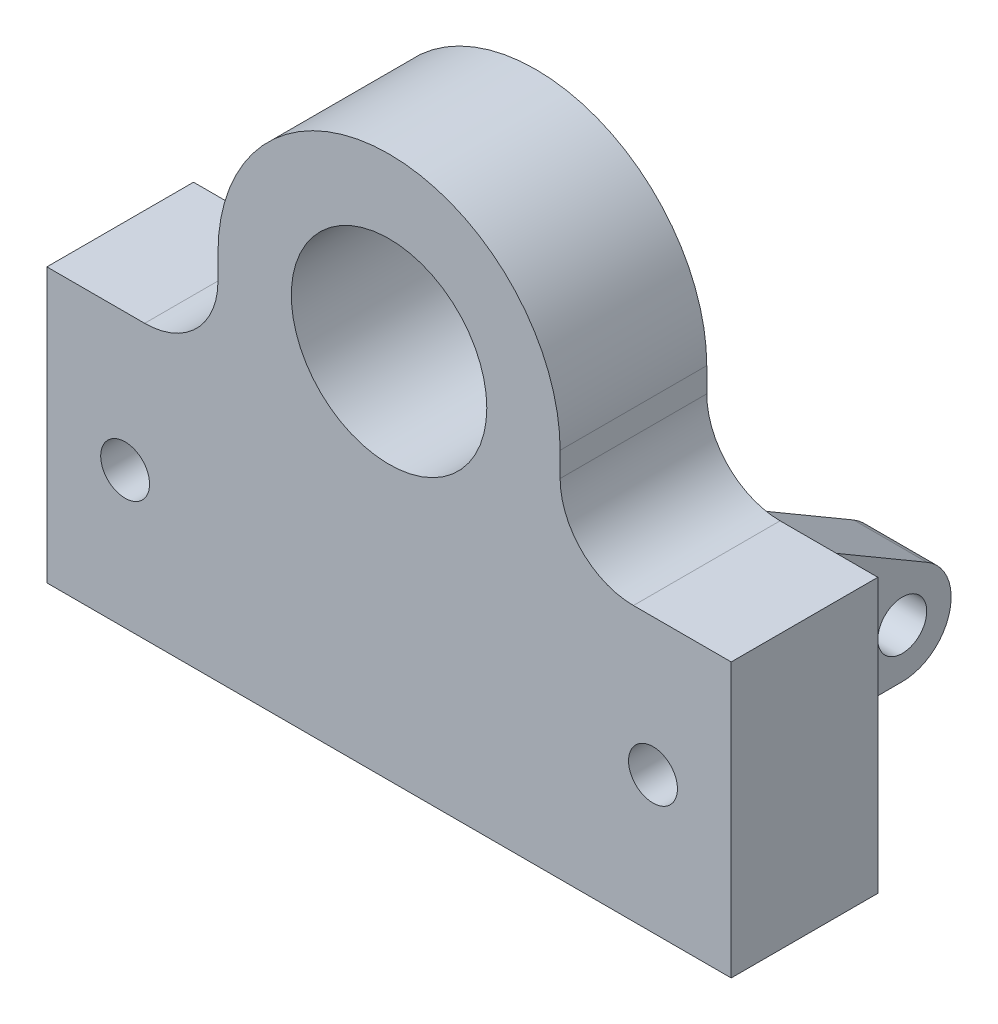
ISO-10303-21;
HEADER;
FILE_DESCRIPTION(('STEP AP214'),'2;1');
FILE_NAME('part.step','',(''),(''),'','','');
FILE_SCHEMA(('AUTOMOTIVE_DESIGN { 1 0 10303 214 1 1 1 1 }'));
ENDSEC;
DATA;
#1=APPLICATION_CONTEXT('core data for automotive mechanical design processes');
#2=APPLICATION_PROTOCOL_DEFINITION('international standard','automotive_design',2000,#1);
#3=PRODUCT_CONTEXT('',#1,'mechanical');
#4=PRODUCT('Part','Part','',(#3));
#5=PRODUCT_RELATED_PRODUCT_CATEGORY('part','',(#4));
#6=PRODUCT_DEFINITION_FORMATION('','',#4);
#7=PRODUCT_DEFINITION_CONTEXT('part definition',#1,'design');
#8=PRODUCT_DEFINITION('design','',#6,#7);
#9=PRODUCT_DEFINITION_SHAPE('','',#8);
#10=(LENGTH_UNIT() NAMED_UNIT(*) SI_UNIT(.MILLI.,.METRE.));
#11=(NAMED_UNIT(*) PLANE_ANGLE_UNIT() SI_UNIT($,.RADIAN.));
#12=(NAMED_UNIT(*) SI_UNIT($,.STERADIAN.) SOLID_ANGLE_UNIT());
#13=UNCERTAINTY_MEASURE_WITH_UNIT(LENGTH_MEASURE(1.E-05),#10,'distance_accuracy_value','');
#14=(GEOMETRIC_REPRESENTATION_CONTEXT(3) GLOBAL_UNCERTAINTY_ASSIGNED_CONTEXT((#13)) GLOBAL_UNIT_ASSIGNED_CONTEXT((#10,
#11,#12)) REPRESENTATION_CONTEXT('',''));
#15=CARTESIAN_POINT('',(0.,0.,0.));
#16=DIRECTION('',(0.,0.,1.));
#17=DIRECTION('',(1.,0.,0.));
#18=AXIS2_PLACEMENT_3D('',#15,#16,#17);
#19=CARTESIAN_POINT('',(0.,0.,30.));
#20=DIRECTION('',(0.,1.,0.));
#21=DIRECTION('',(0.,0.,1.));
#22=AXIS2_PLACEMENT_3D('',#19,#20,#21);
#23=PLANE('',#22);
#24=DIRECTION('',(1.,0.,0.));
#25=VECTOR('',#24,1.);
#26=CARTESIAN_POINT('',(0.,0.,0.));
#27=LINE('',#26,#25);
#28=CARTESIAN_POINT('',(0.,0.,0.));
#29=VERTEX_POINT('',#28);
#30=CARTESIAN_POINT('',(35.,0.,0.));
#31=VERTEX_POINT('',#30);
#32=EDGE_CURVE('E251',#29,#31,#27,.T.);
#33=ORIENTED_EDGE('',*,*,#32,.T.);
#34=DIRECTION('',(0.,0.,-1.));
#35=VECTOR('',#34,1.);
#36=CARTESIAN_POINT('',(35.,0.,0.));
#37=LINE('',#36,#35);
#38=CARTESIAN_POINT('',(35.,0.,-40.));
#39=VERTEX_POINT('',#38);
#40=EDGE_CURVE('E189',#31,#39,#37,.T.);
#41=ORIENTED_EDGE('',*,*,#40,.T.);
#42=DIRECTION('',(-1.,0.,0.));
#43=VECTOR('',#42,1.);
#44=CARTESIAN_POINT('',(50.,0.,-40.));
#45=LINE('',#44,#43);
#46=CARTESIAN_POINT('',(50.,0.,-40.));
#47=VERTEX_POINT('',#46);
#48=EDGE_CURVE('E222',#47,#39,#45,.T.);
#49=ORIENTED_EDGE('',*,*,#48,.F.);
#50=DIRECTION('',(0.,0.,-1.));
#51=VECTOR('',#50,1.);
#52=CARTESIAN_POINT('',(50.,0.,0.));
#53=LINE('',#52,#51);
#54=CARTESIAN_POINT('',(50.,0.,0.));
#55=VERTEX_POINT('',#54);
#56=EDGE_CURVE('E200',#55,#47,#53,.T.);
#57=ORIENTED_EDGE('',*,*,#56,.F.);
#58=CARTESIAN_POINT('',(90.,0.,0.));
#59=VERTEX_POINT('',#58);
#60=EDGE_CURVE('E258',#55,#59,#27,.T.);
#61=ORIENTED_EDGE('',*,*,#60,.T.);
#62=DIRECTION('',(0.,0.,-1.));
#63=VECTOR('',#62,1.);
#64=CARTESIAN_POINT('',(90.,0.,0.));
#65=LINE('',#64,#63);
#66=CARTESIAN_POINT('',(90.,0.,-40.));
#67=VERTEX_POINT('',#66);
#68=EDGE_CURVE('E187',#59,#67,#65,.T.);
#69=ORIENTED_EDGE('',*,*,#68,.T.);
#70=DIRECTION('',(-1.,0.,0.));
#71=VECTOR('',#70,1.);
#72=CARTESIAN_POINT('',(105.,0.,-40.));
#73=LINE('',#72,#71);
#74=CARTESIAN_POINT('',(105.,0.,-40.));
#75=VERTEX_POINT('',#74);
#76=EDGE_CURVE('E175',#75,#67,#73,.T.);
#77=ORIENTED_EDGE('',*,*,#76,.F.);
#78=DIRECTION('',(0.,0.,-1.));
#79=VECTOR('',#78,1.);
#80=CARTESIAN_POINT('',(105.,0.,0.));
#81=LINE('',#80,#79);
#82=CARTESIAN_POINT('',(105.,0.,0.));
#83=VERTEX_POINT('',#82);
#84=EDGE_CURVE('E177',#83,#75,#81,.T.);
#85=ORIENTED_EDGE('',*,*,#84,.F.);
#86=CARTESIAN_POINT('',(140.,0.,0.));
#87=VERTEX_POINT('',#86);
#88=EDGE_CURVE('E64',#83,#87,#27,.T.);
#89=ORIENTED_EDGE('',*,*,#88,.T.);
#90=DIRECTION('',(0.,0.,-1.));
#91=VECTOR('',#90,1.);
#92=CARTESIAN_POINT('',(140.,0.,30.));
#93=LINE('',#92,#91);
#94=CARTESIAN_POINT('',(140.,0.,30.));
#95=VERTEX_POINT('',#94);
#96=EDGE_CURVE('E11',#95,#87,#93,.T.);
#97=ORIENTED_EDGE('',*,*,#96,.F.);
#98=DIRECTION('',(1.,0.,0.));
#99=VECTOR('',#98,1.);
#100=CARTESIAN_POINT('',(0.,0.,30.));
#101=LINE('',#100,#99);
#102=CARTESIAN_POINT('',(0.,0.,30.));
#103=VERTEX_POINT('',#102);
#104=EDGE_CURVE('E229',#103,#95,#101,.T.);
#105=ORIENTED_EDGE('',*,*,#104,.F.);
#106=DIRECTION('',(0.,0.,-1.));
#107=VECTOR('',#106,1.);
#108=CARTESIAN_POINT('',(0.,0.,30.));
#109=LINE('',#108,#107);
#110=EDGE_CURVE('E252',#103,#29,#109,.T.);
#111=ORIENTED_EDGE('',*,*,#110,.T.);
#112=EDGE_LOOP('',(#33,#41,#49,#57,#61,#69,#77,#85,#89,#97,#105,#111));
#113=FACE_BOUND('',#112,.T.);
#114=ADVANCED_FACE('F44',(#113),#23,.F.);
#115=CARTESIAN_POINT('',(140.,0.,30.));
#116=DIRECTION('',(-1.,0.,0.));
#117=DIRECTION('',(0.,0.,1.));
#118=AXIS2_PLACEMENT_3D('',#115,#116,#117);
#119=PLANE('',#118);
#120=DIRECTION('',(0.,1.,0.));
#121=VECTOR('',#120,1.);
#122=CARTESIAN_POINT('',(140.,0.,0.));
#123=LINE('',#122,#121);
#124=CARTESIAN_POINT('',(140.,56.,0.));
#125=VERTEX_POINT('',#124);
#126=EDGE_CURVE('E254',#87,#125,#123,.T.);
#127=ORIENTED_EDGE('',*,*,#126,.T.);
#128=DIRECTION('',(0.,0.,-1.));
#129=VECTOR('',#128,1.);
#130=CARTESIAN_POINT('',(140.,56.,30.));
#131=LINE('',#130,#129);
#132=CARTESIAN_POINT('',(140.,56.,30.));
#133=VERTEX_POINT('',#132);
#134=EDGE_CURVE('E52',#133,#125,#131,.T.);
#135=ORIENTED_EDGE('',*,*,#134,.F.);
#136=DIRECTION('',(0.,1.,0.));
#137=VECTOR('',#136,1.);
#138=CARTESIAN_POINT('',(140.,0.,30.));
#139=LINE('',#138,#137);
#140=EDGE_CURVE('E231',#95,#133,#139,.T.);
#141=ORIENTED_EDGE('',*,*,#140,.F.);
#142=ORIENTED_EDGE('',*,*,#96,.T.);
#143=EDGE_LOOP('',(#127,#135,#141,#142));
#144=FACE_BOUND('',#143,.T.);
#145=ADVANCED_FACE('F302',(#144),#119,.F.);
#146=CARTESIAN_POINT('',(125.,56.,30.));
#147=DIRECTION('',(0.,-1.,0.));
#148=DIRECTION('',(0.,0.,-1.));
#149=AXIS2_PLACEMENT_3D('',#146,#147,#148);
#150=PLANE('',#149);
#151=DIRECTION('',(-1.,0.,0.));
#152=VECTOR('',#151,1.);
#153=CARTESIAN_POINT('',(125.,56.,0.));
#154=LINE('',#153,#152);
#155=CARTESIAN_POINT('',(120.,56.,0.));
#156=VERTEX_POINT('',#155);
#157=EDGE_CURVE('E259',#125,#156,#154,.T.);
#158=ORIENTED_EDGE('',*,*,#157,.T.);
#159=DIRECTION('',(0.,0.,-1.));
#160=VECTOR('',#159,1.);
#161=CARTESIAN_POINT('',(120.,56.,30.));
#162=LINE('',#161,#160);
#163=CARTESIAN_POINT('',(120.,56.,30.));
#164=VERTEX_POINT('',#163);
#165=EDGE_CURVE('E294',#164,#156,#162,.T.);
#166=ORIENTED_EDGE('',*,*,#165,.F.);
#167=DIRECTION('',(-1.,0.,0.));
#168=VECTOR('',#167,1.);
#169=CARTESIAN_POINT('',(140.,56.,30.));
#170=LINE('',#169,#168);
#171=EDGE_CURVE('E237',#133,#164,#170,.T.);
#172=ORIENTED_EDGE('',*,*,#171,.F.);
#173=ORIENTED_EDGE('',*,*,#134,.T.);
#174=EDGE_LOOP('',(#158,#166,#172,#173));
#175=FACE_BOUND('',#174,.T.);
#176=ADVANCED_FACE('F303',(#175),#150,.F.);
#177=CARTESIAN_POINT('',(120.,71.,30.));
#178=DIRECTION('',(0.,0.,-1.));
#179=DIRECTION('',(-1.,0.,0.));
#180=AXIS2_PLACEMENT_3D('',#177,#178,#179);
#181=CYLINDRICAL_SURFACE('',#180,15.);
#182=CARTESIAN_POINT('',(120.,71.,0.));
#183=DIRECTION('',(0.,0.,-1.));
#184=DIRECTION('',(1.,0.,0.));
#185=AXIS2_PLACEMENT_3D('',#182,#183,#184);
#186=CIRCLE('',#185,15.);
#187=CARTESIAN_POINT('',(105.,71.,0.));
#188=VERTEX_POINT('',#187);
#189=EDGE_CURVE('E261',#156,#188,#186,.T.);
#190=ORIENTED_EDGE('',*,*,#189,.T.);
#191=DIRECTION('',(0.,0.,-1.));
#192=VECTOR('',#191,1.);
#193=CARTESIAN_POINT('',(105.,71.,30.));
#194=LINE('',#193,#192);
#195=CARTESIAN_POINT('',(105.,71.,30.));
#196=VERTEX_POINT('',#195);
#197=EDGE_CURVE('E292',#196,#188,#194,.T.);
#198=ORIENTED_EDGE('',*,*,#197,.F.);
#199=CARTESIAN_POINT('',(120.,71.,30.));
#200=DIRECTION('',(0.,0.,-1.));
#201=DIRECTION('',(1.,0.,0.));
#202=AXIS2_PLACEMENT_3D('',#199,#200,#201);
#203=CIRCLE('',#202,15.);
#204=EDGE_CURVE('E236',#164,#196,#203,.T.);
#205=ORIENTED_EDGE('',*,*,#204,.F.);
#206=ORIENTED_EDGE('',*,*,#165,.T.);
#207=EDGE_LOOP('',(#190,#198,#205,#206));
#208=FACE_BOUND('',#207,.T.);
#209=ADVANCED_FACE('F311',(#208),#181,.F.);
#210=CARTESIAN_POINT('',(105.,71.,30.));
#211=DIRECTION('',(-1.,0.,0.));
#212=DIRECTION('',(0.,-1.,0.));
#213=AXIS2_PLACEMENT_3D('',#210,#211,#212);
#214=PLANE('',#213);
#215=DIRECTION('',(0.,1.,0.));
#216=VECTOR('',#215,1.);
#217=CARTESIAN_POINT('',(105.,71.,0.));
#218=LINE('',#217,#216);
#219=CARTESIAN_POINT('',(105.,76.,0.));
#220=VERTEX_POINT('',#219);
#221=EDGE_CURVE('E263',#188,#220,#218,.T.);
#222=ORIENTED_EDGE('',*,*,#221,.T.);
#223=DIRECTION('',(0.,0.,-1.));
#224=VECTOR('',#223,1.);
#225=CARTESIAN_POINT('',(105.,76.,30.));
#226=LINE('',#225,#224);
#227=CARTESIAN_POINT('',(105.,76.,30.));
#228=VERTEX_POINT('',#227);
#229=EDGE_CURVE('E286',#228,#220,#226,.T.);
#230=ORIENTED_EDGE('',*,*,#229,.F.);
#231=DIRECTION('',(0.,1.,0.));
#232=VECTOR('',#231,1.);
#233=CARTESIAN_POINT('',(105.,71.,30.));
#234=LINE('',#233,#232);
#235=EDGE_CURVE('E238',#196,#228,#234,.T.);
#236=ORIENTED_EDGE('',*,*,#235,.F.);
#237=ORIENTED_EDGE('',*,*,#197,.T.);
#238=EDGE_LOOP('',(#222,#230,#236,#237));
#239=FACE_BOUND('',#238,.T.);
#240=ADVANCED_FACE('F320',(#239),#214,.F.);
#241=CARTESIAN_POINT('',(70.,76.,30.));
#242=DIRECTION('',(0.,0.,-1.));
#243=DIRECTION('',(-1.,0.,0.));
#244=AXIS2_PLACEMENT_3D('',#241,#242,#243);
#245=CYLINDRICAL_SURFACE('',#244,35.);
#246=CARTESIAN_POINT('',(70.,76.,0.));
#247=DIRECTION('',(0.,0.,1.));
#248=DIRECTION('',(1.,0.,0.));
#249=AXIS2_PLACEMENT_3D('',#246,#247,#248);
#250=CIRCLE('',#249,35.);
#251=CARTESIAN_POINT('',(35.,76.,0.));
#252=VERTEX_POINT('',#251);
#253=EDGE_CURVE('E264',#220,#252,#250,.T.);
#254=ORIENTED_EDGE('',*,*,#253,.T.);
#255=DIRECTION('',(0.,0.,-1.));
#256=VECTOR('',#255,1.);
#257=CARTESIAN_POINT('',(35.,76.,30.));
#258=LINE('',#257,#256);
#259=CARTESIAN_POINT('',(35.,76.,30.));
#260=VERTEX_POINT('',#259);
#261=EDGE_CURVE('E284',#260,#252,#258,.T.);
#262=ORIENTED_EDGE('',*,*,#261,.F.);
#263=CARTESIAN_POINT('',(70.,76.,30.));
#264=DIRECTION('',(0.,0.,1.));
#265=DIRECTION('',(1.,0.,0.));
#266=AXIS2_PLACEMENT_3D('',#263,#264,#265);
#267=CIRCLE('',#266,35.);
#268=EDGE_CURVE('E245',#228,#260,#267,.T.);
#269=ORIENTED_EDGE('',*,*,#268,.F.);
#270=ORIENTED_EDGE('',*,*,#229,.T.);
#271=EDGE_LOOP('',(#254,#262,#269,#270));
#272=FACE_BOUND('',#271,.T.);
#273=ADVANCED_FACE('F405',(#272),#245,.T.);
#274=CARTESIAN_POINT('',(35.,71.,30.));
#275=DIRECTION('',(1.,0.,0.));
#276=DIRECTION('',(0.,1.,0.));
#277=AXIS2_PLACEMENT_3D('',#274,#275,#276);
#278=PLANE('',#277);
#279=DIRECTION('',(0.,-1.,0.));
#280=VECTOR('',#279,1.);
#281=CARTESIAN_POINT('',(35.,71.,0.));
#282=LINE('',#281,#280);
#283=CARTESIAN_POINT('',(35.,71.,0.));
#284=VERTEX_POINT('',#283);
#285=EDGE_CURVE('E270',#252,#284,#282,.T.);
#286=ORIENTED_EDGE('',*,*,#285,.T.);
#287=DIRECTION('',(0.,0.,-1.));
#288=VECTOR('',#287,1.);
#289=CARTESIAN_POINT('',(35.,71.,30.));
#290=LINE('',#289,#288);
#291=CARTESIAN_POINT('',(35.,71.,30.));
#292=VERTEX_POINT('',#291);
#293=EDGE_CURVE('E285',#292,#284,#290,.T.);
#294=ORIENTED_EDGE('',*,*,#293,.F.);
#295=DIRECTION('',(0.,-1.,0.));
#296=VECTOR('',#295,1.);
#297=CARTESIAN_POINT('',(35.,71.,30.));
#298=LINE('',#297,#296);
#299=EDGE_CURVE('E242',#260,#292,#298,.T.);
#300=ORIENTED_EDGE('',*,*,#299,.F.);
#301=ORIENTED_EDGE('',*,*,#261,.T.);
#302=EDGE_LOOP('',(#286,#294,#300,#301));
#303=FACE_BOUND('',#302,.T.);
#304=ADVANCED_FACE('F403',(#303),#278,.F.);
#305=CARTESIAN_POINT('',(20.,71.,30.));
#306=DIRECTION('',(0.,0.,-1.));
#307=DIRECTION('',(-1.,0.,0.));
#308=AXIS2_PLACEMENT_3D('',#305,#306,#307);
#309=CYLINDRICAL_SURFACE('',#308,15.);
#310=CARTESIAN_POINT('',(20.,71.,0.));
#311=DIRECTION('',(0.,0.,-1.));
#312=DIRECTION('',(1.,0.,0.));
#313=AXIS2_PLACEMENT_3D('',#310,#311,#312);
#314=CIRCLE('',#313,15.);
#315=CARTESIAN_POINT('',(20.,56.,0.));
#316=VERTEX_POINT('',#315);
#317=EDGE_CURVE('E267',#284,#316,#314,.T.);
#318=ORIENTED_EDGE('',*,*,#317,.T.);
#319=DIRECTION('',(0.,0.,-1.));
#320=VECTOR('',#319,1.);
#321=CARTESIAN_POINT('',(20.,56.,30.));
#322=LINE('',#321,#320);
#323=CARTESIAN_POINT('',(20.,56.,30.));
#324=VERTEX_POINT('',#323);
#325=EDGE_CURVE('E276',#324,#316,#322,.T.);
#326=ORIENTED_EDGE('',*,*,#325,.F.);
#327=CARTESIAN_POINT('',(20.,71.,30.));
#328=DIRECTION('',(0.,0.,-1.));
#329=DIRECTION('',(1.,0.,0.));
#330=AXIS2_PLACEMENT_3D('',#327,#328,#329);
#331=CIRCLE('',#330,15.);
#332=EDGE_CURVE('E248',#292,#324,#331,.T.);
#333=ORIENTED_EDGE('',*,*,#332,.F.);
#334=ORIENTED_EDGE('',*,*,#293,.T.);
#335=EDGE_LOOP('',(#318,#326,#333,#334));
#336=FACE_BOUND('',#335,.T.);
#337=ADVANCED_FACE('F407',(#336),#309,.F.);
#338=CARTESIAN_POINT('',(0.,56.,30.));
#339=DIRECTION('',(0.,-1.,0.));
#340=DIRECTION('',(0.,0.,-1.));
#341=AXIS2_PLACEMENT_3D('',#338,#339,#340);
#342=PLANE('',#341);
#343=DIRECTION('',(-1.,0.,0.));
#344=VECTOR('',#343,1.);
#345=CARTESIAN_POINT('',(0.,56.,0.));
#346=LINE('',#345,#344);
#347=CARTESIAN_POINT('',(0.,56.,0.));
#348=VERTEX_POINT('',#347);
#349=EDGE_CURVE('E271',#316,#348,#346,.T.);
#350=ORIENTED_EDGE('',*,*,#349,.T.);
#351=DIRECTION('',(0.,0.,-1.));
#352=VECTOR('',#351,1.);
#353=CARTESIAN_POINT('',(0.,56.,30.));
#354=LINE('',#353,#352);
#355=CARTESIAN_POINT('',(0.,56.,30.));
#356=VERTEX_POINT('',#355);
#357=EDGE_CURVE('E277',#356,#348,#354,.T.);
#358=ORIENTED_EDGE('',*,*,#357,.F.);
#359=DIRECTION('',(-1.,0.,0.));
#360=VECTOR('',#359,1.);
#361=CARTESIAN_POINT('',(0.,56.,30.));
#362=LINE('',#361,#360);
#363=EDGE_CURVE('E246',#324,#356,#362,.T.);
#364=ORIENTED_EDGE('',*,*,#363,.F.);
#365=ORIENTED_EDGE('',*,*,#325,.T.);
#366=EDGE_LOOP('',(#350,#358,#364,#365));
#367=FACE_BOUND('',#366,.T.);
#368=ADVANCED_FACE('F411',(#367),#342,.F.);
#369=CARTESIAN_POINT('',(0.,0.,30.));
#370=DIRECTION('',(1.,0.,0.));
#371=DIRECTION('',(0.,0.,-1.));
#372=AXIS2_PLACEMENT_3D('',#369,#370,#371);
#373=PLANE('',#372);
#374=DIRECTION('',(0.,-1.,0.));
#375=VECTOR('',#374,1.);
#376=CARTESIAN_POINT('',(0.,0.,0.));
#377=LINE('',#376,#375);
#378=EDGE_CURVE('E232',#348,#29,#377,.T.);
#379=ORIENTED_EDGE('',*,*,#378,.T.);
#380=ORIENTED_EDGE('',*,*,#110,.F.);
#381=DIRECTION('',(0.,-1.,0.));
#382=VECTOR('',#381,1.);
#383=CARTESIAN_POINT('',(0.,0.,30.));
#384=LINE('',#383,#382);
#385=EDGE_CURVE('E249',#356,#103,#384,.T.);
#386=ORIENTED_EDGE('',*,*,#385,.F.);
#387=ORIENTED_EDGE('',*,*,#357,.T.);
#388=EDGE_LOOP('',(#379,#380,#386,#387));
#389=FACE_BOUND('',#388,.T.);
#390=ADVANCED_FACE('F417',(#389),#373,.F.);
#391=CARTESIAN_POINT('',(120.,71.,30.));
#392=DIRECTION('',(0.,0.,1.));
#393=DIRECTION('',(1.,0.,0.));
#394=AXIS2_PLACEMENT_3D('',#391,#392,#393);
#395=PLANE('',#394);
#396=CARTESIAN_POINT('',(124.,28.,30.));
#397=DIRECTION('',(0.,0.,1.));
#398=DIRECTION('',(1.,0.,0.));
#399=AXIS2_PLACEMENT_3D('',#396,#397,#398);
#400=CIRCLE('',#399,5.);
#401=CARTESIAN_POINT('',(129.,28.,30.));
#402=VERTEX_POINT('',#401);
#403=EDGE_CURVE('E355',#402,#402,#400,.T.);
#404=ORIENTED_EDGE('',*,*,#403,.F.);
#405=EDGE_LOOP('',(#404));
#406=FACE_BOUND('',#405,.T.);
#407=CARTESIAN_POINT('',(16.,28.,30.));
#408=DIRECTION('',(0.,0.,1.));
#409=DIRECTION('',(1.,0.,0.));
#410=AXIS2_PLACEMENT_3D('',#407,#408,#409);
#411=CIRCLE('',#410,5.);
#412=CARTESIAN_POINT('',(21.,28.,30.));
#413=VERTEX_POINT('',#412);
#414=EDGE_CURVE('E360',#413,#413,#411,.T.);
#415=ORIENTED_EDGE('',*,*,#414,.F.);
#416=EDGE_LOOP('',(#415));
#417=FACE_BOUND('',#416,.T.);
#418=CARTESIAN_POINT('',(70.,76.,30.));
#419=DIRECTION('',(0.,0.,1.));
#420=DIRECTION('',(1.,0.,0.));
#421=AXIS2_PLACEMENT_3D('',#418,#419,#420);
#422=CIRCLE('',#421,20.);
#423=CARTESIAN_POINT('',(90.,76.,30.));
#424=VERTEX_POINT('',#423);
#425=EDGE_CURVE('E221',#424,#424,#422,.T.);
#426=ORIENTED_EDGE('',*,*,#425,.F.);
#427=EDGE_LOOP('',(#426));
#428=FACE_BOUND('',#427,.T.);
#429=ORIENTED_EDGE('',*,*,#104,.T.);
#430=ORIENTED_EDGE('',*,*,#140,.T.);
#431=ORIENTED_EDGE('',*,*,#171,.T.);
#432=ORIENTED_EDGE('',*,*,#204,.T.);
#433=ORIENTED_EDGE('',*,*,#235,.T.);
#434=ORIENTED_EDGE('',*,*,#268,.T.);
#435=ORIENTED_EDGE('',*,*,#299,.T.);
#436=ORIENTED_EDGE('',*,*,#332,.T.);
#437=ORIENTED_EDGE('',*,*,#363,.T.);
#438=ORIENTED_EDGE('',*,*,#385,.T.);
#439=EDGE_LOOP('',(#429,#430,#431,#432,#433,#434,#435,#436,#437,#438));
#440=FACE_BOUND('',#439,.T.);
#441=ADVANCED_FACE('F321',(#406,#417,#428,#440),#395,.T.);
#442=CARTESIAN_POINT('',(120.,71.,0.));
#443=DIRECTION('',(0.,0.,1.));
#444=DIRECTION('',(1.,0.,0.));
#445=AXIS2_PLACEMENT_3D('',#442,#443,#444);
#446=PLANE('',#445);
#447=CARTESIAN_POINT('',(124.,28.,0.));
#448=DIRECTION('',(0.,0.,-1.));
#449=DIRECTION('',(-1.,0.,0.));
#450=AXIS2_PLACEMENT_3D('',#447,#448,#449);
#451=CIRCLE('',#450,5.);
#452=CARTESIAN_POINT('',(119.,28.,0.));
#453=VERTEX_POINT('',#452);
#454=EDGE_CURVE('E359',#453,#453,#451,.T.);
#455=ORIENTED_EDGE('',*,*,#454,.F.);
#456=EDGE_LOOP('',(#455));
#457=FACE_BOUND('',#456,.T.);
#458=CARTESIAN_POINT('',(16.,28.,0.));
#459=DIRECTION('',(0.,0.,-1.));
#460=DIRECTION('',(-1.,0.,0.));
#461=AXIS2_PLACEMENT_3D('',#458,#459,#460);
#462=CIRCLE('',#461,5.);
#463=CARTESIAN_POINT('',(11.,28.,0.));
#464=VERTEX_POINT('',#463);
#465=EDGE_CURVE('E363',#464,#464,#462,.T.);
#466=ORIENTED_EDGE('',*,*,#465,.F.);
#467=EDGE_LOOP('',(#466));
#468=FACE_BOUND('',#467,.T.);
#469=ORIENTED_EDGE('',*,*,#88,.F.);
#470=DIRECTION('',(0.,-1.,0.));
#471=VECTOR('',#470,1.);
#472=CARTESIAN_POINT('',(105.,0.,0.));
#473=LINE('',#472,#471);
#474=CARTESIAN_POINT('',(105.,45.,0.));
#475=VERTEX_POINT('',#474);
#476=EDGE_CURVE('E58',#475,#83,#473,.T.);
#477=ORIENTED_EDGE('',*,*,#476,.F.);
#478=DIRECTION('',(-1.,0.,0.));
#479=VECTOR('',#478,1.);
#480=CARTESIAN_POINT('',(105.,45.,0.));
#481=LINE('',#480,#479);
#482=CARTESIAN_POINT('',(90.,45.,0.));
#483=VERTEX_POINT('',#482);
#484=EDGE_CURVE('E194',#475,#483,#481,.T.);
#485=ORIENTED_EDGE('',*,*,#484,.T.);
#486=DIRECTION('',(0.,-1.,0.));
#487=VECTOR('',#486,1.);
#488=CARTESIAN_POINT('',(90.,0.,0.));
#489=LINE('',#488,#487);
#490=EDGE_CURVE('E184',#483,#59,#489,.T.);
#491=ORIENTED_EDGE('',*,*,#490,.T.);
#492=ORIENTED_EDGE('',*,*,#60,.F.);
#493=DIRECTION('',(0.,-1.,0.));
#494=VECTOR('',#493,1.);
#495=CARTESIAN_POINT('',(50.,0.,0.));
#496=LINE('',#495,#494);
#497=CARTESIAN_POINT('',(50.,45.,0.));
#498=VERTEX_POINT('',#497);
#499=EDGE_CURVE('E210',#498,#55,#496,.T.);
#500=ORIENTED_EDGE('',*,*,#499,.F.);
#501=DIRECTION('',(-1.,0.,0.));
#502=VECTOR('',#501,1.);
#503=CARTESIAN_POINT('',(50.,45.,0.));
#504=LINE('',#503,#502);
#505=CARTESIAN_POINT('',(35.,45.,0.));
#506=VERTEX_POINT('',#505);
#507=EDGE_CURVE('E208',#498,#506,#504,.T.);
#508=ORIENTED_EDGE('',*,*,#507,.T.);
#509=DIRECTION('',(0.,-1.,0.));
#510=VECTOR('',#509,1.);
#511=CARTESIAN_POINT('',(35.,0.,0.));
#512=LINE('',#511,#510);
#513=EDGE_CURVE('E201',#506,#31,#512,.T.);
#514=ORIENTED_EDGE('',*,*,#513,.T.);
#515=ORIENTED_EDGE('',*,*,#32,.F.);
#516=ORIENTED_EDGE('',*,*,#378,.F.);
#517=ORIENTED_EDGE('',*,*,#349,.F.);
#518=ORIENTED_EDGE('',*,*,#317,.F.);
#519=ORIENTED_EDGE('',*,*,#285,.F.);
#520=ORIENTED_EDGE('',*,*,#253,.F.);
#521=ORIENTED_EDGE('',*,*,#221,.F.);
#522=ORIENTED_EDGE('',*,*,#189,.F.);
#523=ORIENTED_EDGE('',*,*,#157,.F.);
#524=ORIENTED_EDGE('',*,*,#126,.F.);
#525=EDGE_LOOP('',(#469,#477,#485,#491,#492,#500,#508,#514,#515,#516,#517,#518,#519,#520,#521,
#522,#523,#524));
#526=FACE_BOUND('',#525,.T.);
#527=CARTESIAN_POINT('',(70.,76.,0.));
#528=DIRECTION('',(0.,0.,1.));
#529=DIRECTION('',(1.,0.,0.));
#530=AXIS2_PLACEMENT_3D('',#527,#528,#529);
#531=CIRCLE('',#530,20.);
#532=CARTESIAN_POINT('',(90.,76.,0.));
#533=VERTEX_POINT('',#532);
#534=EDGE_CURVE('E223',#533,#533,#531,.T.);
#535=ORIENTED_EDGE('',*,*,#534,.T.);
#536=EDGE_LOOP('',(#535));
#537=FACE_BOUND('',#536,.T.);
#538=ADVANCED_FACE('F308',(#457,#468,#526,#537),#446,.F.);
#539=CARTESIAN_POINT('',(70.,76.,0.));
#540=DIRECTION('',(0.,0.,1.));
#541=DIRECTION('',(1.,0.,0.));
#542=AXIS2_PLACEMENT_3D('',#539,#540,#541);
#543=CYLINDRICAL_SURFACE('',#542,20.);
#544=ORIENTED_EDGE('',*,*,#534,.F.);
#545=EDGE_LOOP('',(#544));
#546=FACE_BOUND('',#545,.T.);
#547=ORIENTED_EDGE('',*,*,#425,.T.);
#548=EDGE_LOOP('',(#547));
#549=FACE_BOUND('',#548,.T.);
#550=ADVANCED_FACE('F371',(#546,#549),#543,.F.);
#551=CARTESIAN_POINT('',(50.,9.99999999999933,-40.));
#552=DIRECTION('',(-1.,0.,0.));
#553=DIRECTION('',(0.,0.,1.));
#554=AXIS2_PLACEMENT_3D('',#551,#552,#553);
#555=CYLINDRICAL_SURFACE('',#554,9.99999999999933);
#556=CARTESIAN_POINT('',(35.,9.99999999999933,-40.));
#557=DIRECTION('',(1.,0.,0.));
#558=DIRECTION('',(0.,0.,-1.));
#559=AXIS2_PLACEMENT_3D('',#556,#557,#558);
#560=CIRCLE('',#559,9.99999999999933);
#561=CARTESIAN_POINT('',(35.,18.6303054930326,-45.0515173064046));
#562=VERTEX_POINT('',#561);
#563=EDGE_CURVE('E191',#39,#562,#560,.T.);
#564=ORIENTED_EDGE('',*,*,#563,.T.);
#565=DIRECTION('',(-1.,0.,0.));
#566=VECTOR('',#565,1.);
#567=CARTESIAN_POINT('',(50.,18.6303054930326,-45.0515173064046));
#568=LINE('',#567,#566);
#569=CARTESIAN_POINT('',(50.,18.6303054930326,-45.0515173064046));
#570=VERTEX_POINT('',#569);
#571=EDGE_CURVE('E217',#570,#562,#568,.T.);
#572=ORIENTED_EDGE('',*,*,#571,.F.);
#573=CARTESIAN_POINT('',(50.,9.99999999999933,-40.));
#574=DIRECTION('',(1.,0.,0.));
#575=DIRECTION('',(0.,0.,-1.));
#576=AXIS2_PLACEMENT_3D('',#573,#574,#575);
#577=CIRCLE('',#576,9.99999999999933);
#578=EDGE_CURVE('E205',#47,#570,#577,.T.);
#579=ORIENTED_EDGE('',*,*,#578,.F.);
#580=ORIENTED_EDGE('',*,*,#48,.T.);
#581=EDGE_LOOP('',(#564,#572,#579,#580));
#582=FACE_BOUND('',#581,.T.);
#583=ADVANCED_FACE('F430',(#582),#555,.T.);
#584=CARTESIAN_POINT('',(50.,45.,0.));
#585=DIRECTION('',(0.,-0.86303054930339,0.505151730640497));
#586=DIRECTION('',(0.,-0.505151730640497,-0.86303054930339));
#587=AXIS2_PLACEMENT_3D('',#584,#585,#586);
#588=PLANE('',#587);
#589=DIRECTION('',(0.,0.505151730640497,0.86303054930339));
#590=VECTOR('',#589,1.);
#591=CARTESIAN_POINT('',(35.,45.,0.));
#592=LINE('',#591,#590);
#593=EDGE_CURVE('E211',#562,#506,#592,.T.);
#594=ORIENTED_EDGE('',*,*,#593,.T.);
#595=ORIENTED_EDGE('',*,*,#507,.F.);
#596=DIRECTION('',(0.,0.505151730640497,0.86303054930339));
#597=VECTOR('',#596,1.);
#598=CARTESIAN_POINT('',(50.,45.,0.));
#599=LINE('',#598,#597);
#600=EDGE_CURVE('E202',#570,#498,#599,.T.);
#601=ORIENTED_EDGE('',*,*,#600,.F.);
#602=ORIENTED_EDGE('',*,*,#571,.T.);
#603=EDGE_LOOP('',(#594,#595,#601,#602));
#604=FACE_BOUND('',#603,.T.);
#605=ADVANCED_FACE('F431',(#604),#588,.F.);
#606=CARTESIAN_POINT('',(50.,9.99999999999933,-40.));
#607=DIRECTION('',(1.,0.,0.));
#608=DIRECTION('',(0.,0.,-1.));
#609=AXIS2_PLACEMENT_3D('',#606,#607,#608);
#610=PLANE('',#609);
#611=CARTESIAN_POINT('',(50.,9.99999999999933,-40.));
#612=DIRECTION('',(1.,0.,0.));
#613=DIRECTION('',(0.,0.,-1.));
#614=AXIS2_PLACEMENT_3D('',#611,#612,#613);
#615=CIRCLE('',#614,5.0000000000002);
#616=CARTESIAN_POINT('',(50.,9.99999999999933,-45.0000000000002));
#617=VERTEX_POINT('',#616);
#618=EDGE_CURVE('E333',#617,#617,#615,.T.);
#619=ORIENTED_EDGE('',*,*,#618,.F.);
#620=EDGE_LOOP('',(#619));
#621=FACE_BOUND('',#620,.T.);
#622=ORIENTED_EDGE('',*,*,#56,.T.);
#623=ORIENTED_EDGE('',*,*,#578,.T.);
#624=ORIENTED_EDGE('',*,*,#600,.T.);
#625=ORIENTED_EDGE('',*,*,#499,.T.);
#626=EDGE_LOOP('',(#622,#623,#624,#625));
#627=FACE_BOUND('',#626,.T.);
#628=ADVANCED_FACE('F434',(#621,#627),#610,.T.);
#629=CARTESIAN_POINT('',(35.,9.99999999999933,-40.));
#630=DIRECTION('',(1.,0.,0.));
#631=DIRECTION('',(0.,0.,-1.));
#632=AXIS2_PLACEMENT_3D('',#629,#630,#631);
#633=PLANE('',#632);
#634=CARTESIAN_POINT('',(35.,9.99999999999933,-40.));
#635=DIRECTION('',(1.,0.,0.));
#636=DIRECTION('',(0.,0.,-1.));
#637=AXIS2_PLACEMENT_3D('',#634,#635,#636);
#638=CIRCLE('',#637,5.0000000000002);
#639=CARTESIAN_POINT('',(35.,9.99999999999933,-45.0000000000002));
#640=VERTEX_POINT('',#639);
#641=EDGE_CURVE('E353',#640,#640,#638,.T.);
#642=ORIENTED_EDGE('',*,*,#641,.T.);
#643=EDGE_LOOP('',(#642));
#644=FACE_BOUND('',#643,.T.);
#645=ORIENTED_EDGE('',*,*,#40,.F.);
#646=ORIENTED_EDGE('',*,*,#513,.F.);
#647=ORIENTED_EDGE('',*,*,#593,.F.);
#648=ORIENTED_EDGE('',*,*,#563,.F.);
#649=EDGE_LOOP('',(#645,#646,#647,#648));
#650=FACE_BOUND('',#649,.T.);
#651=ADVANCED_FACE('F440',(#644,#650),#633,.F.);
#652=CARTESIAN_POINT('',(105.,9.99999999999933,-40.));
#653=DIRECTION('',(-1.,0.,0.));
#654=DIRECTION('',(0.,0.,1.));
#655=AXIS2_PLACEMENT_3D('',#652,#653,#654);
#656=CYLINDRICAL_SURFACE('',#655,9.99999999999933);
#657=CARTESIAN_POINT('',(90.,9.99999999999933,-40.));
#658=DIRECTION('',(1.,0.,0.));
#659=DIRECTION('',(0.,0.,-1.));
#660=AXIS2_PLACEMENT_3D('',#657,#658,#659);
#661=CIRCLE('',#660,9.99999999999933);
#662=CARTESIAN_POINT('',(90.,18.6303054930326,-45.0515173064046));
#663=VERTEX_POINT('',#662);
#664=EDGE_CURVE('E331',#67,#663,#661,.T.);
#665=ORIENTED_EDGE('',*,*,#664,.T.);
#666=DIRECTION('',(-1.,0.,0.));
#667=VECTOR('',#666,1.);
#668=CARTESIAN_POINT('',(105.,18.6303054930326,-45.0515173064046));
#669=LINE('',#668,#667);
#670=CARTESIAN_POINT('',(105.,18.6303054930326,-45.0515173064046));
#671=VERTEX_POINT('',#670);
#672=EDGE_CURVE('E174',#671,#663,#669,.T.);
#673=ORIENTED_EDGE('',*,*,#672,.F.);
#674=CARTESIAN_POINT('',(105.,9.99999999999933,-40.));
#675=DIRECTION('',(1.,0.,0.));
#676=DIRECTION('',(0.,0.,-1.));
#677=AXIS2_PLACEMENT_3D('',#674,#675,#676);
#678=CIRCLE('',#677,9.99999999999933);
#679=EDGE_CURVE('E169',#75,#671,#678,.T.);
#680=ORIENTED_EDGE('',*,*,#679,.F.);
#681=ORIENTED_EDGE('',*,*,#76,.T.);
#682=EDGE_LOOP('',(#665,#673,#680,#681));
#683=FACE_BOUND('',#682,.T.);
#684=ADVANCED_FACE('F168',(#683),#656,.T.);
#685=CARTESIAN_POINT('',(105.,45.,0.));
#686=DIRECTION('',(0.,-0.86303054930339,0.505151730640497));
#687=DIRECTION('',(0.,-0.505151730640497,-0.86303054930339));
#688=AXIS2_PLACEMENT_3D('',#685,#686,#687);
#689=PLANE('',#688);
#690=DIRECTION('',(0.,0.505151730640497,0.86303054930339));
#691=VECTOR('',#690,1.);
#692=CARTESIAN_POINT('',(90.,45.,0.));
#693=LINE('',#692,#691);
#694=EDGE_CURVE('E340',#663,#483,#693,.T.);
#695=ORIENTED_EDGE('',*,*,#694,.T.);
#696=ORIENTED_EDGE('',*,*,#484,.F.);
#697=DIRECTION('',(0.,0.505151730640497,0.86303054930339));
#698=VECTOR('',#697,1.);
#699=CARTESIAN_POINT('',(105.,45.,0.));
#700=LINE('',#699,#698);
#701=EDGE_CURVE('E176',#671,#475,#700,.T.);
#702=ORIENTED_EDGE('',*,*,#701,.F.);
#703=ORIENTED_EDGE('',*,*,#672,.T.);
#704=EDGE_LOOP('',(#695,#696,#702,#703));
#705=FACE_BOUND('',#704,.T.);
#706=ADVANCED_FACE('F448',(#705),#689,.F.);
#707=CARTESIAN_POINT('',(105.,9.99999999999933,-40.));
#708=DIRECTION('',(1.,0.,0.));
#709=DIRECTION('',(0.,0.,-1.));
#710=AXIS2_PLACEMENT_3D('',#707,#708,#709);
#711=PLANE('',#710);
#712=CARTESIAN_POINT('',(105.,9.99999999999933,-40.));
#713=DIRECTION('',(1.,0.,0.));
#714=DIRECTION('',(0.,0.,-1.));
#715=AXIS2_PLACEMENT_3D('',#712,#713,#714);
#716=CIRCLE('',#715,5.0000000000002);
#717=CARTESIAN_POINT('',(105.,9.99999999999933,-45.0000000000002));
#718=VERTEX_POINT('',#717);
#719=EDGE_CURVE('E346',#718,#718,#716,.T.);
#720=ORIENTED_EDGE('',*,*,#719,.F.);
#721=EDGE_LOOP('',(#720));
#722=FACE_BOUND('',#721,.T.);
#723=ORIENTED_EDGE('',*,*,#84,.T.);
#724=ORIENTED_EDGE('',*,*,#679,.T.);
#725=ORIENTED_EDGE('',*,*,#701,.T.);
#726=ORIENTED_EDGE('',*,*,#476,.T.);
#727=EDGE_LOOP('',(#723,#724,#725,#726));
#728=FACE_BOUND('',#727,.T.);
#729=ADVANCED_FACE('F185',(#722,#728),#711,.T.);
#730=CARTESIAN_POINT('',(90.,9.99999999999933,-40.));
#731=DIRECTION('',(1.,0.,0.));
#732=DIRECTION('',(0.,0.,-1.));
#733=AXIS2_PLACEMENT_3D('',#730,#731,#732);
#734=PLANE('',#733);
#735=CARTESIAN_POINT('',(90.,9.99999999999933,-40.));
#736=DIRECTION('',(1.,0.,0.));
#737=DIRECTION('',(0.,0.,-1.));
#738=AXIS2_PLACEMENT_3D('',#735,#736,#737);
#739=CIRCLE('',#738,5.0000000000002);
#740=CARTESIAN_POINT('',(90.,9.99999999999933,-45.0000000000002));
#741=VERTEX_POINT('',#740);
#742=EDGE_CURVE('E48',#741,#741,#739,.T.);
#743=ORIENTED_EDGE('',*,*,#742,.T.);
#744=EDGE_LOOP('',(#743));
#745=FACE_BOUND('',#744,.T.);
#746=ORIENTED_EDGE('',*,*,#68,.F.);
#747=ORIENTED_EDGE('',*,*,#490,.F.);
#748=ORIENTED_EDGE('',*,*,#694,.F.);
#749=ORIENTED_EDGE('',*,*,#664,.F.);
#750=EDGE_LOOP('',(#746,#747,#748,#749));
#751=FACE_BOUND('',#750,.T.);
#752=ADVANCED_FACE('F335',(#745,#751),#734,.F.);
#753=CARTESIAN_POINT('',(35.,9.99999999999933,-40.));
#754=DIRECTION('',(1.,0.,0.));
#755=DIRECTION('',(0.,0.,-1.));
#756=AXIS2_PLACEMENT_3D('',#753,#754,#755);
#757=CYLINDRICAL_SURFACE('',#756,5.0000000000002);
#758=ORIENTED_EDGE('',*,*,#719,.T.);
#759=EDGE_LOOP('',(#758));
#760=FACE_BOUND('',#759,.T.);
#761=ORIENTED_EDGE('',*,*,#742,.F.);
#762=EDGE_LOOP('',(#761));
#763=FACE_BOUND('',#762,.T.);
#764=ADVANCED_FACE('F387',(#760,#763),#757,.F.);
#765=ORIENTED_EDGE('',*,*,#618,.T.);
#766=EDGE_LOOP('',(#765));
#767=FACE_BOUND('',#766,.T.);
#768=ORIENTED_EDGE('',*,*,#641,.F.);
#769=EDGE_LOOP('',(#768));
#770=FACE_BOUND('',#769,.T.);
#771=ADVANCED_FACE('F380',(#767,#770),#757,.F.);
#772=CARTESIAN_POINT('',(16.,28.,70.));
#773=DIRECTION('',(0.,0.,-1.));
#774=DIRECTION('',(-1.,0.,0.));
#775=AXIS2_PLACEMENT_3D('',#772,#773,#774);
#776=CYLINDRICAL_SURFACE('',#775,5.);
#777=ORIENTED_EDGE('',*,*,#414,.T.);
#778=EDGE_LOOP('',(#777));
#779=FACE_BOUND('',#778,.T.);
#780=ORIENTED_EDGE('',*,*,#465,.T.);
#781=EDGE_LOOP('',(#780));
#782=FACE_BOUND('',#781,.T.);
#783=ADVANCED_FACE('F374',(#779,#782),#776,.F.);
#784=CARTESIAN_POINT('',(124.,28.,70.));
#785=DIRECTION('',(0.,0.,-1.));
#786=DIRECTION('',(-1.,0.,0.));
#787=AXIS2_PLACEMENT_3D('',#784,#785,#786);
#788=CYLINDRICAL_SURFACE('',#787,5.);
#789=ORIENTED_EDGE('',*,*,#403,.T.);
#790=EDGE_LOOP('',(#789));
#791=FACE_BOUND('',#790,.T.);
#792=ORIENTED_EDGE('',*,*,#454,.T.);
#793=EDGE_LOOP('',(#792));
#794=FACE_BOUND('',#793,.T.);
#795=ADVANCED_FACE('F370',(#791,#794),#788,.F.);
#796=CLOSED_SHELL('',(#114,#145,#176,#209,#240,#273,#304,#337,#368,#390,#441,#538,#550,#583,
#605,#628,#651,#684,#706,#729,#752,#764,#771,#783,#795));
#797=MANIFOLD_SOLID_BREP('B2',#796);
#798=ADVANCED_BREP_SHAPE_REPRESENTATION('',(#18,#797),#14);
#799=SHAPE_DEFINITION_REPRESENTATION(#9,#798);
ENDSEC;
END-ISO-10303-21;
